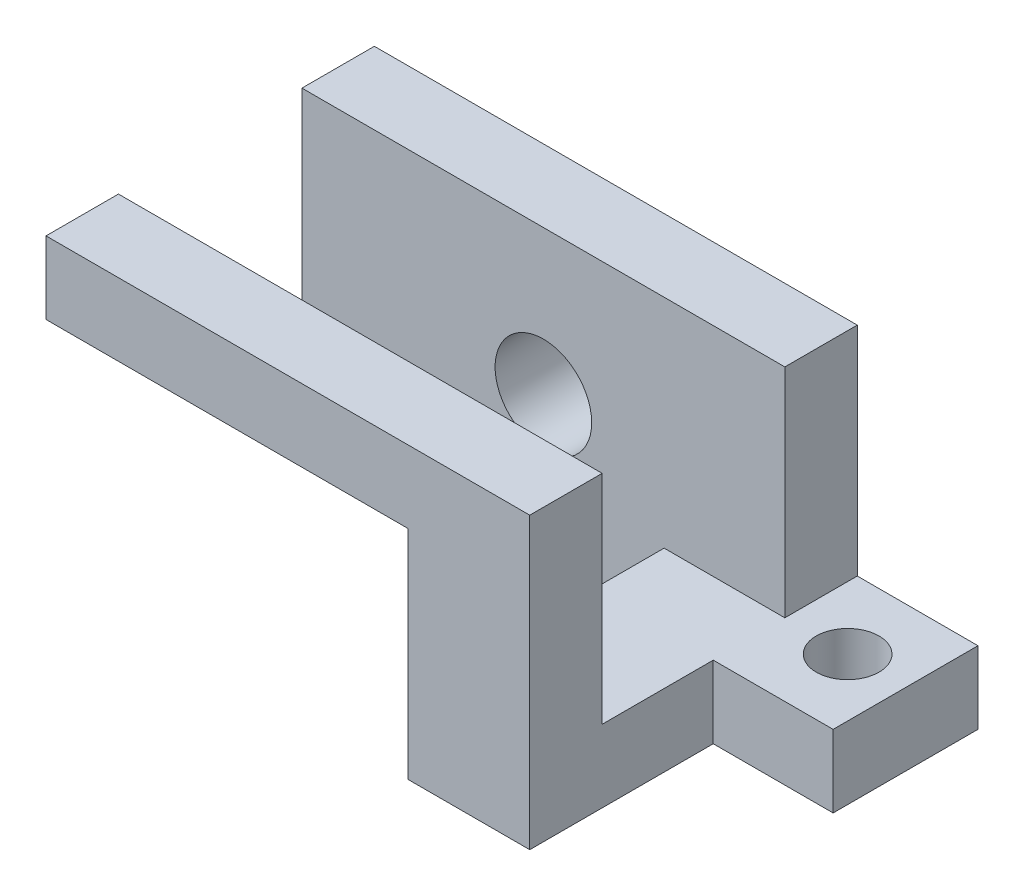
ISO-10303-21;
HEADER;
FILE_DESCRIPTION(('STEP AP214'),'2;1');
FILE_NAME('part.step','',(''),(''),'','','');
FILE_SCHEMA(('AUTOMOTIVE_DESIGN { 1 0 10303 214 1 1 1 1 }'));
ENDSEC;
DATA;
#1=APPLICATION_CONTEXT('core data for automotive mechanical design processes');
#2=APPLICATION_PROTOCOL_DEFINITION('international standard','automotive_design',2000,#1);
#3=PRODUCT_CONTEXT('',#1,'mechanical');
#4=PRODUCT('Part','Part','',(#3));
#5=PRODUCT_RELATED_PRODUCT_CATEGORY('part','',(#4));
#6=PRODUCT_DEFINITION_FORMATION('','',#4);
#7=PRODUCT_DEFINITION_CONTEXT('part definition',#1,'design');
#8=PRODUCT_DEFINITION('design','',#6,#7);
#9=PRODUCT_DEFINITION_SHAPE('','',#8);
#10=(LENGTH_UNIT() NAMED_UNIT(*) SI_UNIT(.MILLI.,.METRE.));
#11=(NAMED_UNIT(*) PLANE_ANGLE_UNIT() SI_UNIT($,.RADIAN.));
#12=(NAMED_UNIT(*) SI_UNIT($,.STERADIAN.) SOLID_ANGLE_UNIT());
#13=UNCERTAINTY_MEASURE_WITH_UNIT(LENGTH_MEASURE(1.E-05),#10,'distance_accuracy_value','');
#14=(GEOMETRIC_REPRESENTATION_CONTEXT(3) GLOBAL_UNCERTAINTY_ASSIGNED_CONTEXT((#13)) GLOBAL_UNIT_ASSIGNED_CONTEXT((#10,
#11,#12)) REPRESENTATION_CONTEXT('',''));
#15=CARTESIAN_POINT('',(0.,0.,0.));
#16=DIRECTION('',(0.,0.,1.));
#17=DIRECTION('',(1.,0.,0.));
#18=AXIS2_PLACEMENT_3D('',#15,#16,#17);
#19=CARTESIAN_POINT('',(25.,-30.,30.));
#20=DIRECTION('',(-1.,0.,0.));
#21=DIRECTION('',(0.,-1.,0.));
#22=AXIS2_PLACEMENT_3D('',#19,#20,#21);
#23=PLANE('',#22);
#24=DIRECTION('',(0.,-1.,0.));
#25=VECTOR('',#24,1.);
#26=CARTESIAN_POINT('',(25.,-30.,68.));
#27=LINE('',#26,#25);
#28=CARTESIAN_POINT('',(25.,15.,68.));
#29=VERTEX_POINT('',#28);
#30=CARTESIAN_POINT('',(25.,-30.,68.));
#31=VERTEX_POINT('',#30);
#32=EDGE_CURVE('E192',#29,#31,#27,.T.);
#33=ORIENTED_EDGE('',*,*,#32,.F.);
#34=DIRECTION('',(0.,0.,1.));
#35=VECTOR('',#34,1.);
#36=CARTESIAN_POINT('',(25.,15.,53.));
#37=LINE('',#36,#35);
#38=CARTESIAN_POINT('',(25.,15.,53.));
#39=VERTEX_POINT('',#38);
#40=EDGE_CURVE('E165',#39,#29,#37,.T.);
#41=ORIENTED_EDGE('',*,*,#40,.F.);
#42=DIRECTION('',(0.,-1.,0.));
#43=VECTOR('',#42,1.);
#44=CARTESIAN_POINT('',(25.,30.,53.));
#45=LINE('',#44,#43);
#46=CARTESIAN_POINT('',(25.,-15.,53.));
#47=VERTEX_POINT('',#46);
#48=EDGE_CURVE('E169',#39,#47,#45,.T.);
#49=ORIENTED_EDGE('',*,*,#48,.T.);
#50=DIRECTION('',(0.,0.,-1.));
#51=VECTOR('',#50,1.);
#52=CARTESIAN_POINT('',(25.,-15.,30.));
#53=LINE('',#52,#51);
#54=CARTESIAN_POINT('',(25.,-15.,15.));
#55=VERTEX_POINT('',#54);
#56=EDGE_CURVE('E61',#47,#55,#53,.T.);
#57=ORIENTED_EDGE('',*,*,#56,.T.);
#58=DIRECTION('',(0.,1.,0.));
#59=VECTOR('',#58,1.);
#60=CARTESIAN_POINT('',(25.,0.,15.));
#61=LINE('',#60,#59);
#62=CARTESIAN_POINT('',(25.,-30.,15.));
#63=VERTEX_POINT('',#62);
#64=EDGE_CURVE('E213',#63,#55,#61,.T.);
#65=ORIENTED_EDGE('',*,*,#64,.F.);
#66=DIRECTION('',(0.,0.,-1.));
#67=VECTOR('',#66,1.);
#68=CARTESIAN_POINT('',(25.,-30.,30.));
#69=LINE('',#68,#67);
#70=EDGE_CURVE('E206',#31,#63,#69,.T.);
#71=ORIENTED_EDGE('',*,*,#70,.F.);
#72=EDGE_LOOP('',(#33,#41,#49,#57,#65,#71));
#73=FACE_BOUND('',#72,.T.);
#74=ADVANCED_FACE('F39',(#73),#23,.T.);
#75=CARTESIAN_POINT('',(25.,-15.,30.));
#76=DIRECTION('',(0.,1.,0.));
#77=DIRECTION('',(-1.,0.,0.));
#78=AXIS2_PLACEMENT_3D('',#75,#76,#77);
#79=PLANE('',#78);
#80=CARTESIAN_POINT('',(63.,-15.,15.));
#81=DIRECTION('',(0.,1.,0.));
#82=DIRECTION('',(-1.,0.,0.));
#83=AXIS2_PLACEMENT_3D('',#80,#81,#82);
#84=CIRCLE('',#83,6.5);
#85=CARTESIAN_POINT('',(56.5,-15.,15.));
#86=VERTEX_POINT('',#85);
#87=EDGE_CURVE('E254',#86,#86,#84,.T.);
#88=ORIENTED_EDGE('',*,*,#87,.F.);
#89=EDGE_LOOP('',(#88));
#90=FACE_BOUND('',#89,.T.);
#91=ORIENTED_EDGE('',*,*,#56,.F.);
#92=DIRECTION('',(-1.,0.,0.));
#93=VECTOR('',#92,1.);
#94=CARTESIAN_POINT('',(25.,-15.,53.));
#95=LINE('',#94,#93);
#96=CARTESIAN_POINT('',(50.1744112780762,-15.,53.));
#97=VERTEX_POINT('',#96);
#98=EDGE_CURVE('E167',#97,#47,#95,.T.);
#99=ORIENTED_EDGE('',*,*,#98,.F.);
#100=DIRECTION('',(0.,0.,-1.));
#101=VECTOR('',#100,1.);
#102=CARTESIAN_POINT('',(50.1744112780762,-15.,68.));
#103=LINE('',#102,#101);
#104=CARTESIAN_POINT('',(50.1744112780762,-15.,30.));
#105=VERTEX_POINT('',#104);
#106=EDGE_CURVE('E194',#97,#105,#103,.T.);
#107=ORIENTED_EDGE('',*,*,#106,.T.);
#108=DIRECTION('',(1.,0.,0.));
#109=VECTOR('',#108,1.);
#110=CARTESIAN_POINT('',(25.,-15.,30.));
#111=LINE('',#110,#109);
#112=CARTESIAN_POINT('',(75.,-15.,30.));
#113=VERTEX_POINT('',#112);
#114=EDGE_CURVE('E205',#105,#113,#111,.T.);
#115=ORIENTED_EDGE('',*,*,#114,.T.);
#116=DIRECTION('',(0.,0.,-1.));
#117=VECTOR('',#116,1.);
#118=CARTESIAN_POINT('',(75.,-15.,30.));
#119=LINE('',#118,#117);
#120=CARTESIAN_POINT('',(75.,-15.,0.));
#121=VERTEX_POINT('',#120);
#122=EDGE_CURVE('E216',#113,#121,#119,.T.);
#123=ORIENTED_EDGE('',*,*,#122,.T.);
#124=DIRECTION('',(1.,0.,0.));
#125=VECTOR('',#124,1.);
#126=CARTESIAN_POINT('',(25.,-15.,0.));
#127=LINE('',#126,#125);
#128=CARTESIAN_POINT('',(50.,-15.,0.));
#129=VERTEX_POINT('',#128);
#130=EDGE_CURVE('E198',#129,#121,#127,.T.);
#131=ORIENTED_EDGE('',*,*,#130,.F.);
#132=DIRECTION('',(0.,0.,-1.));
#133=VECTOR('',#132,1.);
#134=CARTESIAN_POINT('',(50.,-15.,15.));
#135=LINE('',#134,#133);
#136=CARTESIAN_POINT('',(50.,-15.,15.));
#137=VERTEX_POINT('',#136);
#138=EDGE_CURVE('E227',#137,#129,#135,.T.);
#139=ORIENTED_EDGE('',*,*,#138,.F.);
#140=DIRECTION('',(1.,0.,0.));
#141=VECTOR('',#140,1.);
#142=CARTESIAN_POINT('',(0.,-15.,15.));
#143=LINE('',#142,#141);
#144=EDGE_CURVE('E224',#55,#137,#143,.T.);
#145=ORIENTED_EDGE('',*,*,#144,.F.);
#146=EDGE_LOOP('',(#91,#99,#107,#115,#123,#131,#139,#145));
#147=FACE_BOUND('',#146,.T.);
#148=ADVANCED_FACE('F274',(#90,#147),#79,.T.);
#149=CARTESIAN_POINT('',(50.,-30.,15.));
#150=DIRECTION('',(-1.,0.,0.));
#151=DIRECTION('',(0.,0.,1.));
#152=AXIS2_PLACEMENT_3D('',#149,#150,#151);
#153=PLANE('',#152);
#154=DIRECTION('',(0.,1.,0.));
#155=VECTOR('',#154,1.);
#156=CARTESIAN_POINT('',(50.,-30.,15.));
#157=LINE('',#156,#155);
#158=CARTESIAN_POINT('',(50.,30.,15.));
#159=VERTEX_POINT('',#158);
#160=EDGE_CURVE('E233',#137,#159,#157,.T.);
#161=ORIENTED_EDGE('',*,*,#160,.F.);
#162=ORIENTED_EDGE('',*,*,#138,.T.);
#163=DIRECTION('',(0.,1.,0.));
#164=VECTOR('',#163,1.);
#165=CARTESIAN_POINT('',(50.,-30.,0.));
#166=LINE('',#165,#164);
#167=CARTESIAN_POINT('',(50.,30.,0.));
#168=VERTEX_POINT('',#167);
#169=EDGE_CURVE('E229',#129,#168,#166,.T.);
#170=ORIENTED_EDGE('',*,*,#169,.T.);
#171=DIRECTION('',(0.,0.,-1.));
#172=VECTOR('',#171,1.);
#173=CARTESIAN_POINT('',(50.,30.,15.));
#174=LINE('',#173,#172);
#175=EDGE_CURVE('E11',#159,#168,#174,.T.);
#176=ORIENTED_EDGE('',*,*,#175,.F.);
#177=EDGE_LOOP('',(#161,#162,#170,#176));
#178=FACE_BOUND('',#177,.T.);
#179=ADVANCED_FACE('F41',(#178),#153,.F.);
#180=CARTESIAN_POINT('',(-50.,30.,15.));
#181=DIRECTION('',(0.,-1.,0.));
#182=DIRECTION('',(0.,0.,-1.));
#183=AXIS2_PLACEMENT_3D('',#180,#181,#182);
#184=PLANE('',#183);
#185=DIRECTION('',(-1.,0.,0.));
#186=VECTOR('',#185,1.);
#187=CARTESIAN_POINT('',(-50.,30.,0.));
#188=LINE('',#187,#186);
#189=CARTESIAN_POINT('',(-50.,30.,0.));
#190=VERTEX_POINT('',#189);
#191=EDGE_CURVE('E243',#168,#190,#188,.T.);
#192=ORIENTED_EDGE('',*,*,#191,.T.);
#193=DIRECTION('',(0.,0.,-1.));
#194=VECTOR('',#193,1.);
#195=CARTESIAN_POINT('',(-50.,30.,15.));
#196=LINE('',#195,#194);
#197=CARTESIAN_POINT('',(-50.,30.,15.));
#198=VERTEX_POINT('',#197);
#199=EDGE_CURVE('E48',#198,#190,#196,.T.);
#200=ORIENTED_EDGE('',*,*,#199,.F.);
#201=DIRECTION('',(-1.,0.,0.));
#202=VECTOR('',#201,1.);
#203=CARTESIAN_POINT('',(-50.,30.,15.));
#204=LINE('',#203,#202);
#205=EDGE_CURVE('E231',#159,#198,#204,.T.);
#206=ORIENTED_EDGE('',*,*,#205,.F.);
#207=ORIENTED_EDGE('',*,*,#175,.T.);
#208=EDGE_LOOP('',(#192,#200,#206,#207));
#209=FACE_BOUND('',#208,.T.);
#210=ADVANCED_FACE('F296',(#209),#184,.F.);
#211=CARTESIAN_POINT('',(-50.,-30.,15.));
#212=DIRECTION('',(1.,0.,0.));
#213=DIRECTION('',(0.,0.,-1.));
#214=AXIS2_PLACEMENT_3D('',#211,#212,#213);
#215=PLANE('',#214);
#216=DIRECTION('',(0.,-1.,0.));
#217=VECTOR('',#216,1.);
#218=CARTESIAN_POINT('',(-50.,-30.,0.));
#219=LINE('',#218,#217);
#220=CARTESIAN_POINT('',(-50.,-30.,0.));
#221=VERTEX_POINT('',#220);
#222=EDGE_CURVE('E244',#190,#221,#219,.T.);
#223=ORIENTED_EDGE('',*,*,#222,.T.);
#224=DIRECTION('',(0.,0.,-1.));
#225=VECTOR('',#224,1.);
#226=CARTESIAN_POINT('',(-50.,-30.,15.));
#227=LINE('',#226,#225);
#228=CARTESIAN_POINT('',(-50.,-30.,15.));
#229=VERTEX_POINT('',#228);
#230=EDGE_CURVE('E241',#229,#221,#227,.T.);
#231=ORIENTED_EDGE('',*,*,#230,.F.);
#232=DIRECTION('',(0.,-1.,0.));
#233=VECTOR('',#232,1.);
#234=CARTESIAN_POINT('',(-50.,-30.,15.));
#235=LINE('',#234,#233);
#236=EDGE_CURVE('E236',#198,#229,#235,.T.);
#237=ORIENTED_EDGE('',*,*,#236,.F.);
#238=ORIENTED_EDGE('',*,*,#199,.T.);
#239=EDGE_LOOP('',(#223,#231,#237,#238));
#240=FACE_BOUND('',#239,.T.);
#241=ADVANCED_FACE('F310',(#240),#215,.F.);
#242=CARTESIAN_POINT('',(-50.,-30.,15.));
#243=DIRECTION('',(0.,1.,0.));
#244=DIRECTION('',(0.,0.,1.));
#245=AXIS2_PLACEMENT_3D('',#242,#243,#244);
#246=PLANE('',#245);
#247=CARTESIAN_POINT('',(63.,-30.,15.));
#248=DIRECTION('',(0.,1.,0.));
#249=DIRECTION('',(0.,0.,1.));
#250=AXIS2_PLACEMENT_3D('',#247,#248,#249);
#251=CIRCLE('',#250,6.5);
#252=CARTESIAN_POINT('',(63.,-30.,21.5));
#253=VERTEX_POINT('',#252);
#254=EDGE_CURVE('E252',#253,#253,#251,.T.);
#255=ORIENTED_EDGE('',*,*,#254,.T.);
#256=EDGE_LOOP('',(#255));
#257=FACE_BOUND('',#256,.T.);
#258=DIRECTION('',(1.,0.,0.));
#259=VECTOR('',#258,1.);
#260=CARTESIAN_POINT('',(-50.,-30.,0.));
#261=LINE('',#260,#259);
#262=CARTESIAN_POINT('',(75.,-30.,0.));
#263=VERTEX_POINT('',#262);
#264=EDGE_CURVE('E234',#221,#263,#261,.T.);
#265=ORIENTED_EDGE('',*,*,#264,.T.);
#266=DIRECTION('',(0.,0.,-1.));
#267=VECTOR('',#266,1.);
#268=CARTESIAN_POINT('',(75.,-30.,30.));
#269=LINE('',#268,#267);
#270=CARTESIAN_POINT('',(75.,-30.,30.));
#271=VERTEX_POINT('',#270);
#272=EDGE_CURVE('E215',#271,#263,#269,.T.);
#273=ORIENTED_EDGE('',*,*,#272,.F.);
#274=DIRECTION('',(-1.,0.,0.));
#275=VECTOR('',#274,1.);
#276=CARTESIAN_POINT('',(25.,-30.,30.));
#277=LINE('',#276,#275);
#278=CARTESIAN_POINT('',(50.1744112780762,-30.,30.));
#279=VERTEX_POINT('',#278);
#280=EDGE_CURVE('E200',#271,#279,#277,.T.);
#281=ORIENTED_EDGE('',*,*,#280,.T.);
#282=DIRECTION('',(0.,0.,-1.));
#283=VECTOR('',#282,1.);
#284=CARTESIAN_POINT('',(50.1744112780762,-30.,68.));
#285=LINE('',#284,#283);
#286=CARTESIAN_POINT('',(50.1744112780762,-30.,68.));
#287=VERTEX_POINT('',#286);
#288=EDGE_CURVE('E196',#287,#279,#285,.T.);
#289=ORIENTED_EDGE('',*,*,#288,.F.);
#290=DIRECTION('',(1.,0.,0.));
#291=VECTOR('',#290,1.);
#292=CARTESIAN_POINT('',(25.,-30.,68.));
#293=LINE('',#292,#291);
#294=EDGE_CURVE('E187',#31,#287,#293,.T.);
#295=ORIENTED_EDGE('',*,*,#294,.F.);
#296=ORIENTED_EDGE('',*,*,#70,.T.);
#297=DIRECTION('',(1.,0.,0.));
#298=VECTOR('',#297,1.);
#299=CARTESIAN_POINT('',(-50.,-30.,15.));
#300=LINE('',#299,#298);
#301=EDGE_CURVE('E238',#229,#63,#300,.T.);
#302=ORIENTED_EDGE('',*,*,#301,.F.);
#303=ORIENTED_EDGE('',*,*,#230,.T.);
#304=EDGE_LOOP('',(#265,#273,#281,#289,#295,#296,#302,#303));
#305=FACE_BOUND('',#304,.T.);
#306=ADVANCED_FACE('F276',(#257,#305),#246,.F.);
#307=CARTESIAN_POINT('',(0.,0.,15.));
#308=DIRECTION('',(0.,0.,-1.));
#309=DIRECTION('',(-1.,0.,0.));
#310=AXIS2_PLACEMENT_3D('',#307,#308,#309);
#311=PLANE('',#310);
#312=CARTESIAN_POINT('',(0.,0.,15.));
#313=DIRECTION('',(0.,0.,1.));
#314=DIRECTION('',(1.,0.,0.));
#315=AXIS2_PLACEMENT_3D('',#312,#313,#314);
#316=CIRCLE('',#315,10.);
#317=CARTESIAN_POINT('',(10.,0.,15.));
#318=VERTEX_POINT('',#317);
#319=EDGE_CURVE('E261',#318,#318,#316,.T.);
#320=ORIENTED_EDGE('',*,*,#319,.F.);
#321=EDGE_LOOP('',(#320));
#322=FACE_BOUND('',#321,.T.);
#323=ORIENTED_EDGE('',*,*,#64,.T.);
#324=ORIENTED_EDGE('',*,*,#144,.T.);
#325=ORIENTED_EDGE('',*,*,#160,.T.);
#326=ORIENTED_EDGE('',*,*,#205,.T.);
#327=ORIENTED_EDGE('',*,*,#236,.T.);
#328=ORIENTED_EDGE('',*,*,#301,.T.);
#329=EDGE_LOOP('',(#323,#324,#325,#326,#327,#328));
#330=FACE_BOUND('',#329,.T.);
#331=ADVANCED_FACE('F301',(#322,#330),#311,.F.);
#332=CARTESIAN_POINT('',(0.,0.,0.));
#333=DIRECTION('',(0.,0.,-1.));
#334=DIRECTION('',(-1.,0.,0.));
#335=AXIS2_PLACEMENT_3D('',#332,#333,#334);
#336=PLANE('',#335);
#337=CARTESIAN_POINT('',(0.,0.,0.));
#338=DIRECTION('',(0.,0.,-1.));
#339=DIRECTION('',(-1.,0.,0.));
#340=AXIS2_PLACEMENT_3D('',#337,#338,#339);
#341=CIRCLE('',#340,10.);
#342=CARTESIAN_POINT('',(-10.,0.,0.));
#343=VERTEX_POINT('',#342);
#344=EDGE_CURVE('E43',#343,#343,#341,.T.);
#345=ORIENTED_EDGE('',*,*,#344,.F.);
#346=EDGE_LOOP('',(#345));
#347=FACE_BOUND('',#346,.T.);
#348=ORIENTED_EDGE('',*,*,#169,.F.);
#349=ORIENTED_EDGE('',*,*,#130,.T.);
#350=DIRECTION('',(0.,-1.,0.));
#351=VECTOR('',#350,1.);
#352=CARTESIAN_POINT('',(75.,-30.,0.));
#353=LINE('',#352,#351);
#354=EDGE_CURVE('E203',#121,#263,#353,.T.);
#355=ORIENTED_EDGE('',*,*,#354,.T.);
#356=ORIENTED_EDGE('',*,*,#264,.F.);
#357=ORIENTED_EDGE('',*,*,#222,.F.);
#358=ORIENTED_EDGE('',*,*,#191,.F.);
#359=EDGE_LOOP('',(#348,#349,#355,#356,#357,#358));
#360=FACE_BOUND('',#359,.T.);
#361=ADVANCED_FACE('F292',(#347,#360),#336,.T.);
#362=CARTESIAN_POINT('',(75.,-30.,30.));
#363=DIRECTION('',(1.,0.,0.));
#364=DIRECTION('',(0.,0.,-1.));
#365=AXIS2_PLACEMENT_3D('',#362,#363,#364);
#366=PLANE('',#365);
#367=ORIENTED_EDGE('',*,*,#354,.F.);
#368=ORIENTED_EDGE('',*,*,#122,.F.);
#369=DIRECTION('',(0.,-1.,0.));
#370=VECTOR('',#369,1.);
#371=CARTESIAN_POINT('',(75.,-30.,30.));
#372=LINE('',#371,#370);
#373=EDGE_CURVE('E201',#113,#271,#372,.T.);
#374=ORIENTED_EDGE('',*,*,#373,.T.);
#375=ORIENTED_EDGE('',*,*,#272,.T.);
#376=EDGE_LOOP('',(#367,#368,#374,#375));
#377=FACE_BOUND('',#376,.T.);
#378=ADVANCED_FACE('F285',(#377),#366,.T.);
#379=CARTESIAN_POINT('',(0.,0.,30.));
#380=DIRECTION('',(0.,0.,1.));
#381=DIRECTION('',(1.,0.,0.));
#382=AXIS2_PLACEMENT_3D('',#379,#380,#381);
#383=PLANE('',#382);
#384=DIRECTION('',(0.,1.,0.));
#385=VECTOR('',#384,1.);
#386=CARTESIAN_POINT('',(50.1744112780762,-30.,30.));
#387=LINE('',#386,#385);
#388=EDGE_CURVE('E57',#279,#105,#387,.T.);
#389=ORIENTED_EDGE('',*,*,#388,.F.);
#390=ORIENTED_EDGE('',*,*,#280,.F.);
#391=ORIENTED_EDGE('',*,*,#373,.F.);
#392=ORIENTED_EDGE('',*,*,#114,.F.);
#393=EDGE_LOOP('',(#389,#390,#391,#392));
#394=FACE_BOUND('',#393,.T.);
#395=ADVANCED_FACE('F281',(#394),#383,.T.);
#396=CARTESIAN_POINT('',(50.1744112780762,-30.,68.));
#397=DIRECTION('',(-1.,0.,0.));
#398=DIRECTION('',(0.,-1.,0.));
#399=AXIS2_PLACEMENT_3D('',#396,#397,#398);
#400=PLANE('',#399);
#401=ORIENTED_EDGE('',*,*,#388,.T.);
#402=ORIENTED_EDGE('',*,*,#106,.F.);
#403=DIRECTION('',(0.,-1.,0.));
#404=VECTOR('',#403,1.);
#405=CARTESIAN_POINT('',(50.1744112780762,30.,53.));
#406=LINE('',#405,#404);
#407=CARTESIAN_POINT('',(50.1744112780762,30.,53.));
#408=VERTEX_POINT('',#407);
#409=EDGE_CURVE('E183',#408,#97,#406,.T.);
#410=ORIENTED_EDGE('',*,*,#409,.F.);
#411=DIRECTION('',(0.,0.,-1.));
#412=VECTOR('',#411,1.);
#413=CARTESIAN_POINT('',(50.1744112780762,30.,68.));
#414=LINE('',#413,#412);
#415=CARTESIAN_POINT('',(50.1744112780762,30.,68.));
#416=VERTEX_POINT('',#415);
#417=EDGE_CURVE('E177',#416,#408,#414,.T.);
#418=ORIENTED_EDGE('',*,*,#417,.F.);
#419=DIRECTION('',(0.,1.,0.));
#420=VECTOR('',#419,1.);
#421=CARTESIAN_POINT('',(50.1744112780762,-30.,68.));
#422=LINE('',#421,#420);
#423=EDGE_CURVE('E186',#287,#416,#422,.T.);
#424=ORIENTED_EDGE('',*,*,#423,.F.);
#425=ORIENTED_EDGE('',*,*,#288,.T.);
#426=EDGE_LOOP('',(#401,#402,#410,#418,#424,#425));
#427=FACE_BOUND('',#426,.T.);
#428=ADVANCED_FACE('F273',(#427),#400,.F.);
#429=CARTESIAN_POINT('',(0.,0.,68.));
#430=DIRECTION('',(0.,0.,1.));
#431=DIRECTION('',(1.,0.,0.));
#432=AXIS2_PLACEMENT_3D('',#429,#430,#431);
#433=PLANE('',#432);
#434=ORIENTED_EDGE('',*,*,#294,.T.);
#435=ORIENTED_EDGE('',*,*,#423,.T.);
#436=DIRECTION('',(1.,0.,0.));
#437=VECTOR('',#436,1.);
#438=CARTESIAN_POINT('',(25.,30.,68.));
#439=LINE('',#438,#437);
#440=CARTESIAN_POINT('',(-50.,30.,68.));
#441=VERTEX_POINT('',#440);
#442=EDGE_CURVE('E175',#441,#416,#439,.T.);
#443=ORIENTED_EDGE('',*,*,#442,.F.);
#444=DIRECTION('',(0.,1.,0.));
#445=VECTOR('',#444,1.);
#446=CARTESIAN_POINT('',(-50.,30.,68.));
#447=LINE('',#446,#445);
#448=CARTESIAN_POINT('',(-50.,15.,68.));
#449=VERTEX_POINT('',#448);
#450=EDGE_CURVE('E153',#449,#441,#447,.T.);
#451=ORIENTED_EDGE('',*,*,#450,.F.);
#452=DIRECTION('',(1.,0.,0.));
#453=VECTOR('',#452,1.);
#454=CARTESIAN_POINT('',(-50.,15.,68.));
#455=LINE('',#454,#453);
#456=EDGE_CURVE('E148',#449,#29,#455,.T.);
#457=ORIENTED_EDGE('',*,*,#456,.T.);
#458=ORIENTED_EDGE('',*,*,#32,.T.);
#459=EDGE_LOOP('',(#434,#435,#443,#451,#457,#458));
#460=FACE_BOUND('',#459,.T.);
#461=ADVANCED_FACE('F357',(#460),#433,.T.);
#462=CARTESIAN_POINT('',(25.,30.,53.));
#463=DIRECTION('',(0.,0.,1.));
#464=DIRECTION('',(1.,0.,0.));
#465=AXIS2_PLACEMENT_3D('',#462,#463,#464);
#466=PLANE('',#465);
#467=ORIENTED_EDGE('',*,*,#98,.T.);
#468=ORIENTED_EDGE('',*,*,#48,.F.);
#469=DIRECTION('',(1.,0.,0.));
#470=VECTOR('',#469,1.);
#471=CARTESIAN_POINT('',(-50.,15.,53.));
#472=LINE('',#471,#470);
#473=CARTESIAN_POINT('',(-50.,15.,53.));
#474=VERTEX_POINT('',#473);
#475=EDGE_CURVE('E150',#474,#39,#472,.T.);
#476=ORIENTED_EDGE('',*,*,#475,.F.);
#477=DIRECTION('',(0.,-1.,0.));
#478=VECTOR('',#477,1.);
#479=CARTESIAN_POINT('',(-50.,30.,53.));
#480=LINE('',#479,#478);
#481=CARTESIAN_POINT('',(-50.,30.,53.));
#482=VERTEX_POINT('',#481);
#483=EDGE_CURVE('E155',#482,#474,#480,.T.);
#484=ORIENTED_EDGE('',*,*,#483,.F.);
#485=DIRECTION('',(-1.,0.,0.));
#486=VECTOR('',#485,1.);
#487=CARTESIAN_POINT('',(25.,30.,53.));
#488=LINE('',#487,#486);
#489=EDGE_CURVE('E181',#408,#482,#488,.T.);
#490=ORIENTED_EDGE('',*,*,#489,.F.);
#491=ORIENTED_EDGE('',*,*,#409,.T.);
#492=EDGE_LOOP('',(#467,#468,#476,#484,#490,#491));
#493=FACE_BOUND('',#492,.T.);
#494=ADVANCED_FACE('F166',(#493),#466,.F.);
#495=CARTESIAN_POINT('',(0.,30.,0.));
#496=DIRECTION('',(0.,1.,0.));
#497=DIRECTION('',(-1.,0.,0.));
#498=AXIS2_PLACEMENT_3D('',#495,#496,#497);
#499=PLANE('',#498);
#500=ORIENTED_EDGE('',*,*,#442,.T.);
#501=ORIENTED_EDGE('',*,*,#417,.T.);
#502=ORIENTED_EDGE('',*,*,#489,.T.);
#503=DIRECTION('',(0.,0.,-1.));
#504=VECTOR('',#503,1.);
#505=CARTESIAN_POINT('',(-50.,30.,53.));
#506=LINE('',#505,#504);
#507=EDGE_CURVE('E163',#441,#482,#506,.T.);
#508=ORIENTED_EDGE('',*,*,#507,.F.);
#509=EDGE_LOOP('',(#500,#501,#502,#508));
#510=FACE_BOUND('',#509,.T.);
#511=ADVANCED_FACE('F270',(#510),#499,.T.);
#512=CARTESIAN_POINT('',(-50.,15.,53.));
#513=DIRECTION('',(0.,1.,0.));
#514=DIRECTION('',(-1.,0.,0.));
#515=AXIS2_PLACEMENT_3D('',#512,#513,#514);
#516=PLANE('',#515);
#517=ORIENTED_EDGE('',*,*,#40,.T.);
#518=ORIENTED_EDGE('',*,*,#456,.F.);
#519=DIRECTION('',(0.,0.,1.));
#520=VECTOR('',#519,1.);
#521=CARTESIAN_POINT('',(-50.,15.,53.));
#522=LINE('',#521,#520);
#523=EDGE_CURVE('E141',#474,#449,#522,.T.);
#524=ORIENTED_EDGE('',*,*,#523,.F.);
#525=ORIENTED_EDGE('',*,*,#475,.T.);
#526=EDGE_LOOP('',(#517,#518,#524,#525));
#527=FACE_BOUND('',#526,.T.);
#528=ADVANCED_FACE('F143',(#527),#516,.F.);
#529=CARTESIAN_POINT('',(-50.,0.,0.));
#530=DIRECTION('',(-1.,0.,0.));
#531=DIRECTION('',(0.,-1.,0.));
#532=AXIS2_PLACEMENT_3D('',#529,#530,#531);
#533=PLANE('',#532);
#534=ORIENTED_EDGE('',*,*,#483,.T.);
#535=ORIENTED_EDGE('',*,*,#523,.T.);
#536=ORIENTED_EDGE('',*,*,#450,.T.);
#537=ORIENTED_EDGE('',*,*,#507,.T.);
#538=EDGE_LOOP('',(#534,#535,#536,#537));
#539=FACE_BOUND('',#538,.T.);
#540=ADVANCED_FACE('F159',(#539),#533,.T.);
#541=CARTESIAN_POINT('',(63.,-90.,15.));
#542=DIRECTION('',(0.,1.,0.));
#543=DIRECTION('',(-1.,0.,0.));
#544=AXIS2_PLACEMENT_3D('',#541,#542,#543);
#545=CYLINDRICAL_SURFACE('',#544,6.5);
#546=ORIENTED_EDGE('',*,*,#87,.T.);
#547=EDGE_LOOP('',(#546));
#548=FACE_BOUND('',#547,.T.);
#549=ORIENTED_EDGE('',*,*,#254,.F.);
#550=EDGE_LOOP('',(#549));
#551=FACE_BOUND('',#550,.T.);
#552=ADVANCED_FACE('F338',(#548,#551),#545,.F.);
#553=CARTESIAN_POINT('',(0.,0.,-60.));
#554=DIRECTION('',(0.,0.,1.));
#555=DIRECTION('',(1.,0.,0.));
#556=AXIS2_PLACEMENT_3D('',#553,#554,#555);
#557=CYLINDRICAL_SURFACE('',#556,10.);
#558=ORIENTED_EDGE('',*,*,#344,.T.);
#559=EDGE_LOOP('',(#558));
#560=FACE_BOUND('',#559,.T.);
#561=ORIENTED_EDGE('',*,*,#319,.T.);
#562=EDGE_LOOP('',(#561));
#563=FACE_BOUND('',#562,.T.);
#564=ADVANCED_FACE('F336',(#560,#563),#557,.F.);
#565=CLOSED_SHELL('',(#74,#148,#179,#210,#241,#306,#331,#361,#378,#395,#428,#461,#494,#511,#528,
#540,#552,#564));
#566=MANIFOLD_SOLID_BREP('B2',#565);
#567=ADVANCED_BREP_SHAPE_REPRESENTATION('',(#18,#566),#14);
#568=SHAPE_DEFINITION_REPRESENTATION(#9,#567);
ENDSEC;
END-ISO-10303-21;
